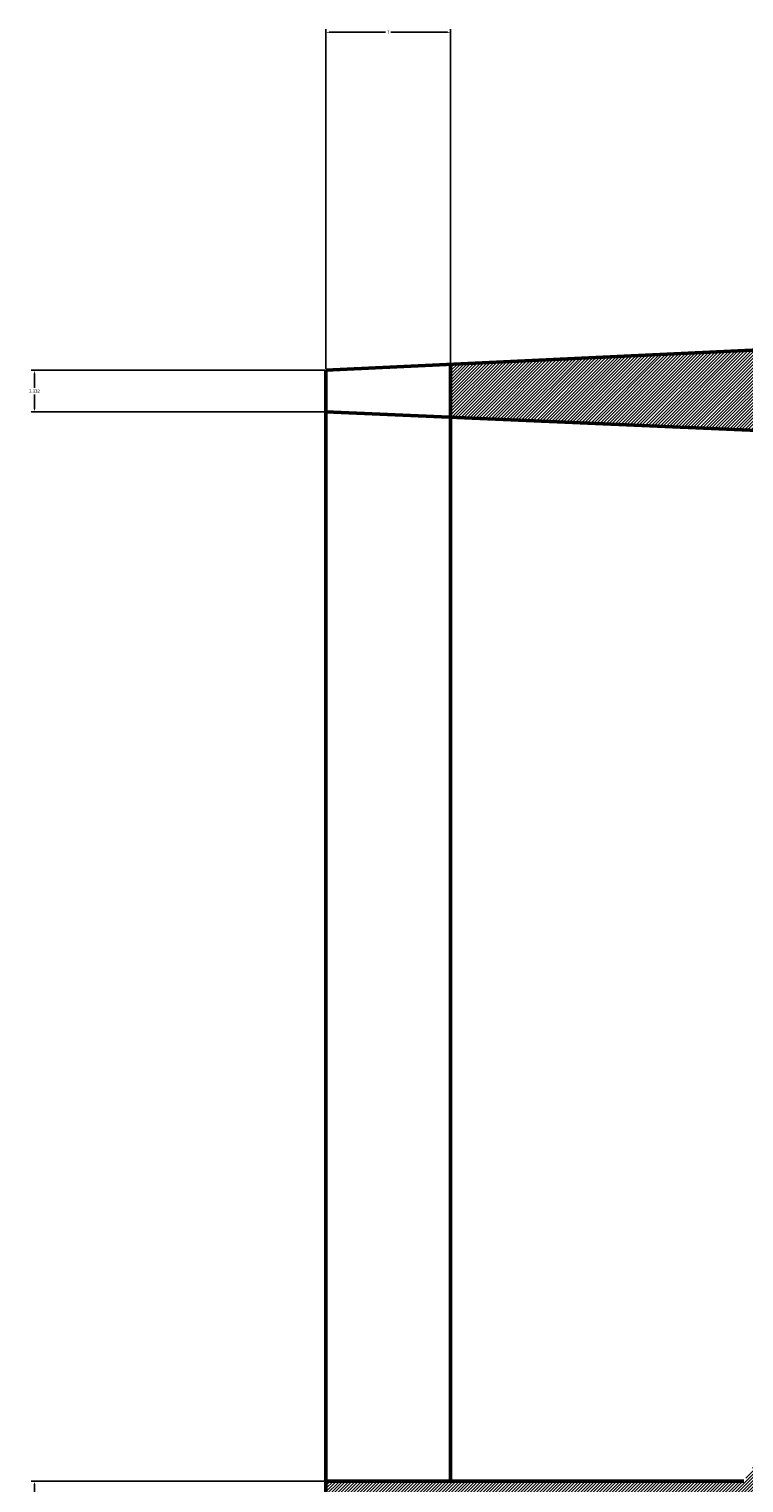
# Model space of a CAD drawing. Units: inches. Extents: x -99 to 284, y -92 to 134.
# Tile 15 of 16: x 187 to 227, y 39 to 120. Entities that reach past the tile are written whole.
import ezdxf

# ---------------------------------------------------------------- set-up
doc = ezdxf.new("R2010")
doc.units = ezdxf.units.IN
doc.header["$MEASUREMENT"] = 0
for name, color, linetype, lineweight in [('M-DIMS', 2, 'Continuous', 18), ('M-HATC', 8, 'Continuous', 18), ('M-OUTL', 7, 'Continuous', 50)]:
    doc.layers.add(name, color=color, linetype=linetype, lineweight=lineweight)
doc.styles.get("Standard").update_dxf_attribs({"font": 'arial.ttf'})
doc.dimstyles.get("Standard").update_dxf_attribs({"dimtxt": 0.18, "dimasz": 0.18, "dimexe": 0.18, "dimexo": 0.0625, "dimgap": 0.09, "dimtad": 0, "dimtih": 1, "dimtoh": 1, "dimdec": 4, "dimzin": 0, "dimdsep": 46, "dimtxsty": 'Standard', "dimcen": 0.09, "dimadec": 0, "dimazin": 0, "dimtfac": 1, "dimtdec": 4, "dimtofl": 0, "dimtmove": 0, "dimatfit": 3, "dimfxl": 1, "dimtolj": 1, "dimtzin": 0, "dimarcsym": 0})

# ---------------------------------------------------------------- blocks, each defined once
blk = doc.blocks.new('*D8')
at = {"layer": 'Defpoints', "color": 0, "transparency": 16777216}
for p in [(210.491, 120.204), (203.491, 101.245), (210.491, 101.573)]:
    blk.add_point(p, dxfattribs=at)
at = {"layer": 'M-DIMS', "color": 0, "lineweight": -2, "transparency": 16777216}
for p, q in [((203.491, 101.307), (203.491, 120.384)), ((203.671, 120.204), (206.843, 120.204)), ((210.311, 120.204), (207.14, 120.204)), ((210.491, 101.636), (210.491, 120.384))]:
    blk.add_line(p, q, dxfattribs=at)
at = {"layer": 'M-DIMS', "color": 0, "transparency": 16777216}
for points in [[(203.671, 120.234), (203.671, 120.174), (203.491, 120.204)], [(210.311, 120.234), (210.311, 120.174), (210.491, 120.204)]]:
    blk.add_solid(points, dxfattribs=at)
at = {"layer": 'M-DIMS', "color": 0, "transparency": 16777216, "insert": (206.991, 120.204), "char_height": 0.18, "attachment_point": 5}
blk.add_mtext('\\A1;7', dxfattribs=at)
blk = doc.blocks.new('*D12')
at = {"layer": 'Defpoints', "color": 0, "transparency": 16777216}
for p in [(187.141, 38.946), (203.491, 38.946), (203.491, -11.467)]:
    blk.add_point(p, dxfattribs=at)
at = {"layer": 'M-DIMS', "color": 0, "lineweight": -2, "transparency": 16777216}
for p, q in [((203.429, 38.946), (186.961, 38.946)), ((187.141, 38.766), (187.141, 13.922)), ((187.141, -11.287), (187.141, 13.558)), ((203.429, -11.467), (186.961, -11.467))]:
    blk.add_line(p, q, dxfattribs=at)
at = {"layer": 'M-DIMS', "color": 0, "transparency": 16777216}
for points in [[(187.111, 38.766), (187.171, 38.766), (187.141, 38.946)], [(187.111, -11.287), (187.171, -11.287), (187.141, -11.467)]]:
    blk.add_solid(points, dxfattribs=at)
at = {"layer": 'M-DIMS', "color": 0, "transparency": 16777216, "insert": (187.141, 13.74), "char_height": 0.18, "attachment_point": 5}
blk.add_mtext('\\A1;50.41', dxfattribs=at)
blk = doc.blocks.new('*D16')
at = {"layer": 'Defpoints', "color": 0, "transparency": 16777216}
for p in [(187.141, 101.245), (203.491, 101.245), (203.491, 98.913)]:
    blk.add_point(p, dxfattribs=at)
at = {"layer": 'M-DIMS', "color": 0, "lineweight": -2, "transparency": 16777216}
for p, q in [((203.429, 101.245), (186.961, 101.245)), ((187.141, 101.065), (187.141, 100.261)), ((187.141, 99.093), (187.141, 99.897)), ((203.429, 98.913), (186.961, 98.913))]:
    blk.add_line(p, q, dxfattribs=at)
at = {"layer": 'M-DIMS', "color": 0, "transparency": 16777216}
for points in [[(187.111, 101.065), (187.171, 101.065), (187.141, 101.245)], [(187.111, 99.093), (187.171, 99.093), (187.141, 98.913)]]:
    blk.add_solid(points, dxfattribs=at)
at = {"layer": 'M-DIMS', "color": 0, "transparency": 16777216, "insert": (187.141, 100.079), "char_height": 0.18, "attachment_point": 5}
blk.add_mtext('\\A1;2.332', dxfattribs=at)

msp = doc.modelspace()

# ---------------------------------------------------------------- hatches: boundary and pattern name
at = {"layer": 'M-HATC'}
h = msp.add_hatch(dxfattribs=at)
h.set_pattern_fill('ANSI31', color=256)
h.set_pattern_definition([(45, (-295.18303, 0), (-0.088388348, 0.088388348), [])])
h.paths.add_polyline_path([(235.9574, 102.7178), (260.4913, 101.5718), (260.4913, 98.6088), (240.4913, 97.7396, -1), (230.4913, 97.7396), (210.4913, 98.6088), (210.4913, 101.573), (235.4326, 102.7424), (235.4913, 102.7396, -0.0233428)])
h.paths.add_polyline_path([(226.9535, 38.946), (203.4913, 38.946), (203.4913, 30.5521), (267.4913, 30.5521), (267.4913, 38.946), (244.0291, 38.946, 0.5614625)])
h.paths.add_polyline_path([(267.4913, 30.5521), (203.4913, 30.5521), (203.4913, 28.5521), (267.4913, 28.5521)])
h.paths.add_polyline_path([(244.0291, -11.4667), (267.4913, -11.4667), (267.4913, -0.9688), (203.4913, -0.9688), (203.4913, -11.4667), (226.9535, -11.4667), (226.9535, -60.8393, -0.294228), (221.0875, -69.9448), (249.6222, -69.8159, -0.2860474), (244.0291, -60.8393)])
h.paths.add_polyline_path([(267.4913, -71.4338), (253.5949, -70.8299, -0.1036016), (249.6222, -69.8159), (221.0875, -69.9448, -0.095981), (217.3877, -70.8299), (203.4913, -71.4338), (203.4913, -73.7656), (235.2571, -75.2549, 0.0117126), (235.4913, -75.2604), (267.4913, -73.7656)])

# ---------------------------------------------------------------- linework, layer by layer
at = {"layer": 'M-OUTL'}
for p, q in [((203.4913, 101.2449), (235.2571, 102.7341)), ((203.4913, 101.2449), (203.4913, 13.7396)), ((203.4913, 101.2449), (203.4913, 97.7396)), ((210.4913, 38.946), (210.4913, 101.573)), ((203.4913, 98.913), (230.4913, 97.7396)), ((226.9535, 38.946), (203.4913, 38.946))]:
    msp.add_line(p, q, dxfattribs=at)

# ---------------------------------------------------------------- dimensions: what is measured, and where the dimension line sits
at = {"layer": 'M-DIMS'}
dim = msp.add_linear_dim(base=(210.4913, 120.2039), p1=(203.4913, 101.2449), p2=(210.4913, 101.573), dimstyle='Standard', override={"dimdec": 0, "dimlfac": 1, "dimrnd": 0, "dimzin": 0, "dimdsep": 46, "dimlunit": 2}, dxfattribs=at)
dim.commit()
dim.dimension.update_dxf_attribs({"geometry": '*D8', "text_midpoint": (206.9913, 120.2039)})
for base, p1, p2, override, picture, middle in [((187.1413, 101.2449), (203.4913, 98.913), (203.4913, 101.2449), {"dimdec": 3, "dimlfac": 1, "dimrnd": 0, "dimzin": 0, "dimdsep": 46, "dimlunit": 2}, '*D16', (187.1413, 100.079)), ((187.1413, 38.946), (203.4913, -11.4667), (203.4913, 38.946), {"dimdec": 2, "dimlfac": 1, "dimrnd": 0, "dimzin": 0, "dimdsep": 46, "dimlunit": 2}, '*D12', (187.1413, 13.7396))]:
    dim = msp.add_linear_dim(base=base, p1=p1, p2=p2, angle=90, dimstyle='Standard', override=override, dxfattribs=at)
    dim.commit()
    dim.dimension.update_dxf_attribs({"geometry": picture, "text_midpoint": middle})

doc.saveas('drawing.dxf')
